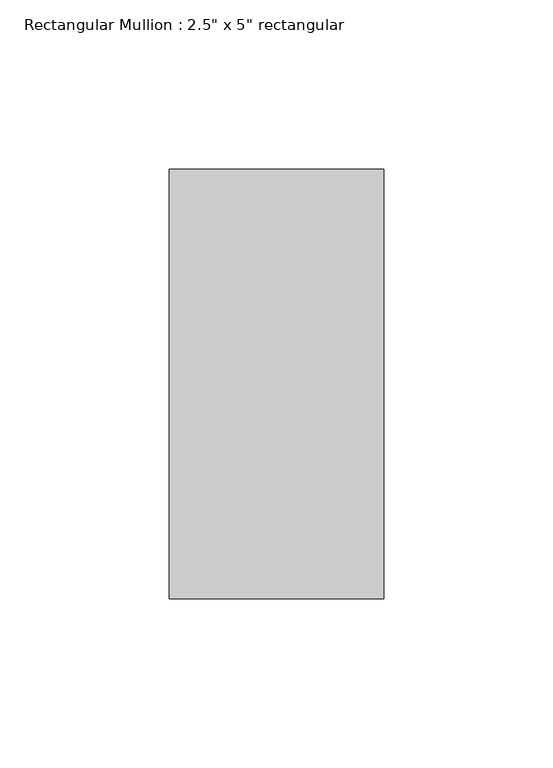
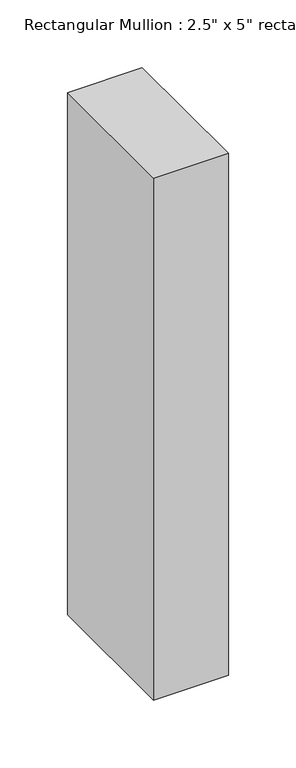
"""IFC4 building model written with IfcOpenShell, lengths in millimetres: member geometry."""

from ifc_helpers import new_model, si_unit, frame, origin, place, context, project, spatial, polyline, outline, extrude, source, transform, mapped, element, save


def member_2b79973d(model_context):
    return source(origin(), model_context, "Body", "SweptSolid", [
        extrude(outline(polyline([(0.0, 63.5), (0.0, -63.5), (-63.5, -63.5), (-63.5, 63.5), (0.0, 63.5)])), frame((0.0, 0.0, -469.9), z_axis=(0.0, 0.0, 1.0), x_axis=(1.0, 0.0, 0.0)), (0.0, 0.0, 1.0), 469.9),
    ])


if __name__ == "__main__":
    model = new_model("IFC4")
    model_context = context("Model", 3, world=origin())
    ifc_project = project(units=[si_unit("LENGTHUNIT", "METRE", prefix="MILLI")], contexts=[model_context])
    site = spatial("IfcSite", under=ifc_project)
    building = spatial("IfcBuilding", under=site)
    placement = place(None, origin())
    member_shape = member_2b79973d(model_context)
    element("IfcMember", 1, ObjectType="Rectangular Mullion : 2.5\" x 5\" rectangular", at=placement, inside=building, context=model_context, shape_type="MappedRepresentation", body=[
        mapped(member_shape, transform((0.0, 0.0, 0.0), x_axis=(1.0, 0.0, 0.0), y_axis=(0.0, 1.0, 0.0), z_axis=(0.0, 0.0, 1.0))),
    ])
    save(model, "model.ifc")

# Revit data of these elements
# Type "Rectangular Mullion : 2.5\" x 5\" rectangular"
#   built-in parameter 1007304 = 0.416667 (stored number, unit not read)
#   built-in parameter 1007301 = 0.104167 (stored number, unit not read)
#   built-in parameter 1007300 = 0.104167 (stored number, unit not read)
# Element 1 (IfcMember, "Rectangular Mullion : 2.5\" x 5\" rectangular")
#   Materials on its faces: "Rectangle 1 sq"
# Materials
#   "Rectangle 1 sq": class "Generic", colour RGB 120 120 120, transparency 0, Cost = 0
